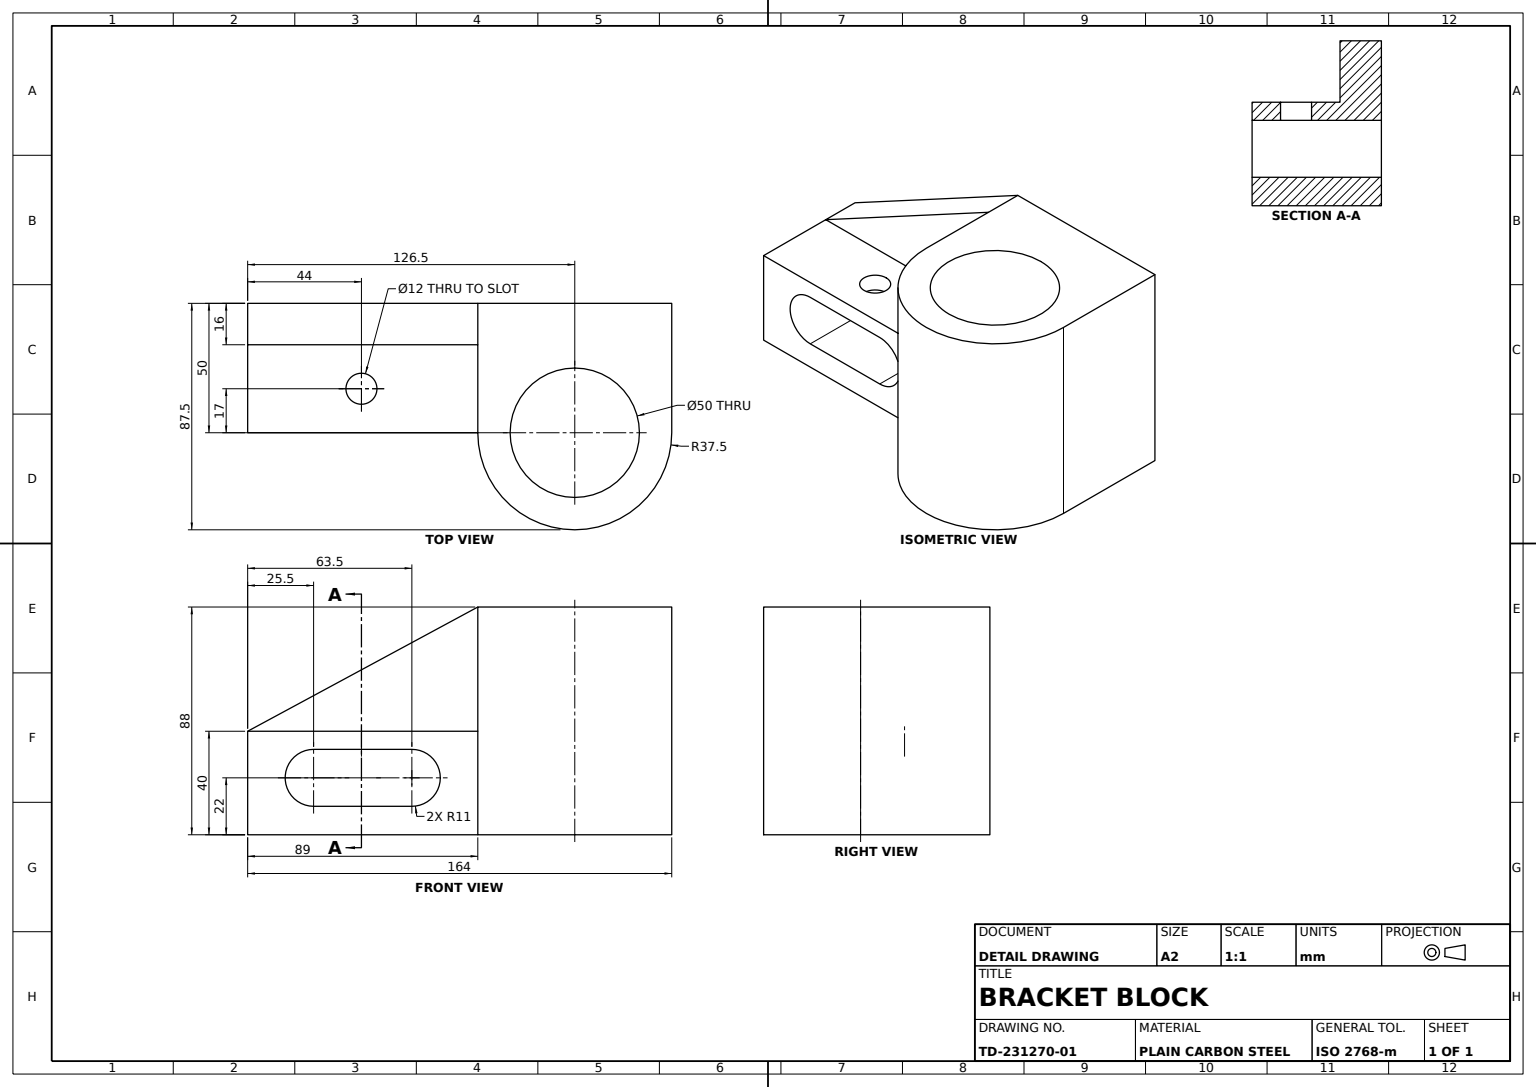
SolidWorks part; units mm, degrees
material "Plain Carbon Steel"
ref_plane "Front Plane" through (0, 0, 0) normal (0, 0, 1) x (1, 0, 0)
ref_plane "Top Plane" through (0, 0, 0) normal (0, 1, 0) x (1, 0, 0)
ref_plane "Right Plane" through (0, 0, 0) normal (1, 0, 0) x (0, 0, -1)
sketch "Base Block Sketch" plane through (0, 0, 0) normal (0, 0, 1) x (1, 0, 0)
  line L0 (0, 0) -> (0, -40)
  line L1 (0, -40) -> (89, -40)
  line L2 (89, -40) -> (89, 0)
  line L3 (89, 0) -> (0, 0)
  dimension "D1" = 89
  dimension "D2" = 40
extrude "Base Block 50mm" add sketch "Base Block Sketch" along normal blind 50
sketch "Rounded Boss Sketch" plane through (0, 0, 0) normal (0, 1, 0) x (1, 0, 0)
  line L0 (89, 0) -> (89, -16)
  line L1 (89, -50) -> (89, 0) construction
  line L3 (164, -16) -> (164, 0)
  line L4 (164, 0) -> (89, 0)
  line L5 (89, -16) -> (89, -50)
  line L6 (164, -16) -> (164, -50)
  line L8 (89, 0) -> (0, 0) construction
  arc A1 (89, -50) -> (164, -50) centre (126.5, -50) ccw
  dimension "D1" = 75
  dimension "D2" = 37.5
  dimension "D3" = 16
extrude "Rounded Boss 44mm" add sketch "Rounded Boss Sketch" against normal blind 44
sketch "Boss Extension Sketch" plane through (0, 0, 0) normal (0, 1, 0) x (1, 0, 0)
  line L0 (164, 0) -> (164, -50)
  line L2 (89, -50) -> (89, 0)
  line L3 (164, 0) -> (0, 0) construction
  line L4 (89, 0) -> (164, 0)
  arc A0 (89, -50) -> (164, -50) centre (126.5, -50) ccw
  dimension "D1" = 75
extrude "Boss Extension 44mm" add sketch "Boss Extension Sketch" along normal blind 44
sketch "Gusset A Sketch" plane through (0, 0, 0) normal (0, 0, -1) x (-1, 0, 0)
  line L0 (-89, 44) -> (-89, 0)
  line L1 (-89, 0) -> (0, 0)
  line L2 (0, 0) -> (-89, 44)
extrude "Gusset A 16mm" add sketch "Gusset A Sketch" against normal blind 16
sketch "Recess Sketch" plane through (0, -44, 0) normal (0, -1, 0) x (1, 0, 0)
  line L0 (89, 0) -> (89, 50)
  line L2 (164, 50) -> (164, 0)
  line L3 (164, 0) -> (89, 0)
  arc A0 (164, 50) -> (89, 50) centre (126.5, 50) ccw
  dimension "D1" = 75
extrude "Recess 4mm" cut sketch "Recess Sketch" against normal blind 4
sketch "Pad Sketch" plane through (0, 44, 0) normal (0, 1, 0) x (1, 0, 0)
  line L0 (89, 0) -> (164, 0)
  line L1 (164, 0) -> (164, -50)
  line L3 (89, -50) -> (89, 0)
  arc A0 (89, -50) -> (164, -50) centre (126.5, -50) ccw
  dimension "D1" = 75
extrude "Pad 4mm" add sketch "Pad Sketch" along normal blind 4
sketch "Gusset B Sketch" plane through (0, 0, 0) normal (0, 0, -1) x (-1, 0, 0)
  line L0 (-89, 48) -> (-89, 44)
  line L1 (-89, 44) -> (0, 0)
  line L2 (0, 0) -> (-89, 48)
extrude "Gusset B 16mm" add sketch "Gusset B Sketch" against normal blind 16
sketch "Bore Sketch Ø50" plane through (0, 48, 0) normal (0, 1, 0) x (1, 0, 0)
  line L1 (89, -16) -> (89, -50) construction
  circle A0 centre (126.5, -50) radius 25
  dimension "D1" = 50
  dimension "D2" = 50
  dimension "D3" = 37.5
extrude "Bore Ø50" cut sketch "Bore Sketch Ø50" against normal blind 88
sketch "Side Slot Sketch" plane through (0, 0, 50) normal (0, 0, 1) x (1, 0, 0)
  line L0 (0, -40) -> (0, -18)
  line L1 (0, 0) -> (0, -40) construction
  line L2 (89, 0) -> (0, 0) construction
  line L6 (25.5, -7) -> (63.5, -7)
  line L7 (25.5, -29) -> (63.5, -29)
  arc A0 (25.5, -7) -> (25.5, -29) centre (25.5, -18) ccw
  arc A1 (63.5, -29) -> (63.5, -7) centre (63.5, -18) ccw
  dimension "D1" = 22
  dimension "D2" = 22
  dimension "D3" = 11
  dimension "D4" = 25.5
  dimension "D5" = 63.5
  dimension "D6" = 18
extrude "Side Slot" cut sketch "Side Slot Sketch" against normal blind 50 contours L7 A1 L6 A0
sketch "Hole Sketch Ø12" plane through (0, 0, 0) normal (0, 1, 0) x (1, 0, 0)
  line L0 (0, -50) -> (0, -16) construction
  line L1 (89, -50) -> (0, -50) construction
  circle A0 centre (44, -33) radius 6
  dimension "D1" = 12
  dimension "D4" = 12
  dimension "D2" = 44
  dimension "D3" = 17
extrude "Hole Ø12" cut sketch "Hole Sketch Ø12" against normal blind 10
